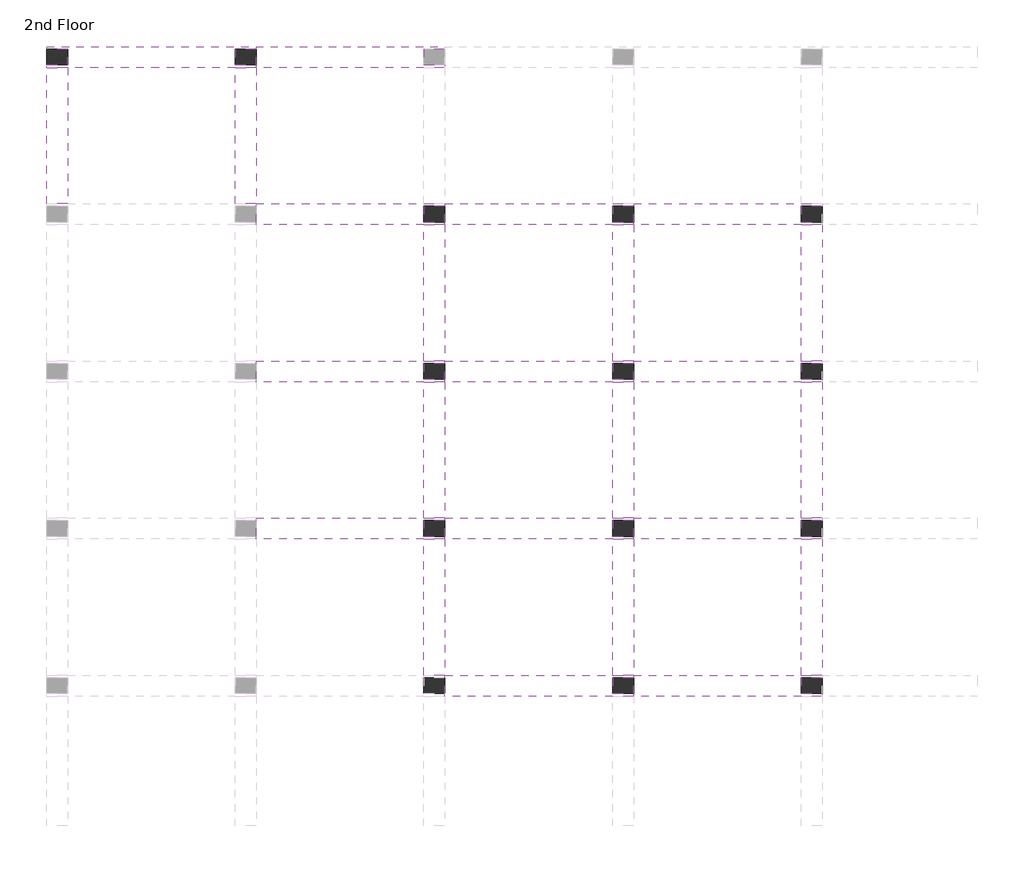
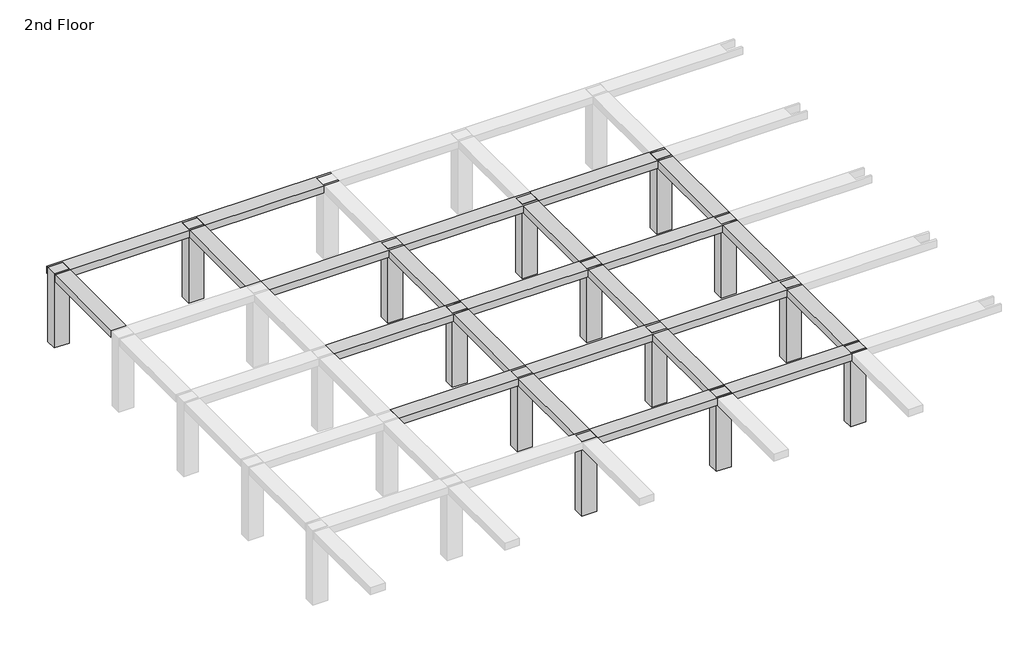
# One storey, part 2 of 3: 24 beams, 14 columns.
"""IFC4 building model written with IfcOpenShell, lengths in millimetres."""

from ifc_helpers import new_model, si_unit, frame, origin, place, context, project, spatial, polyline, outline, extrude, faceted_brep, element, save

model = new_model("IFC4")

# Units and contexts
model_context = context("Model", 3, world=origin())
ifc_project = project(units=[si_unit("LENGTHUNIT", "METRE", prefix="MILLI")], contexts=[model_context])

# Site, building, storey
site = spatial("IfcSite", under=ifc_project)
building = spatial("IfcBuilding", under=site)
storey = spatial("IfcBuildingStorey", under=building, Name="2nd Floor", Elevation=6400.8)

# Beams
placement = place(None, origin())
element("IfcBeam", 1, ObjectType="Concrete-Rectangular Beam : 2' x2'", at=placement, inside=storey, context=model_context, shape_type="Brep", body=[
    faceted_brep([(-5646.474232, 1680.7831222, 9601.2), (-6256.074232, 1680.7831222, 9601.2), (-11132.874232, 1680.7831222, 9601.2), (-11132.874232, 1604.5831222, 9601.2), (-11132.874232, 1147.3831222, 9601.2), (-11132.874232, 1071.1831222, 9601.2), (-6256.074232, 1071.1831222, 9601.2), (-5646.474232, 1071.1831222, 9601.2), (-5646.474232, 1147.3831222, 9601.2), (-6256.074232, 1147.3831222, 9601.2), (-6256.074232, 1604.5831222, 9601.2), (-5646.474232, 1604.5831222, 9601.2), (-5646.474232, 1071.1831222, 9296.4), (-11132.874232, 1071.1831222, 9296.4), (-6256.074232, 1071.1831222, 9296.4), (-11132.874232, 1147.3831222, 9296.4), (-11132.874232, 1604.5831222, 9296.4), (-11132.874232, 1680.7831222, 9296.4), (-6256.074232, 1680.7831222, 9296.4), (-5646.474232, 1680.7831222, 9296.4), (-5646.474232, 1604.5831222, 9296.4), (-6256.074232, 1604.5831222, 9296.4), (-6256.074232, 1147.3831222, 9296.4), (-5646.474232, 1147.3831222, 9296.4)], [[[0, 1, 2, 3, 4, 5, 6, 7, 8, 9, 10, 11]], [[12, 7, 6, 5, 13, 14]], [[12, 14, 13, 15, 16, 17, 18, 19, 20, 21, 22, 23]], [[0, 19, 18, 17, 2, 1]], [[7, 12, 23, 8]], [[5, 4, 3, 2, 17, 16, 15, 13]], [[22, 9, 8, 23]], [[9, 22, 21, 10]], [[10, 21, 20, 11]], [[19, 0, 11, 20]]]),
])
element("IfcBeam", 2, ObjectType="Concrete-Rectangular Beam : 2' x2'", at=placement, inside=storey, context=model_context, shape_type="Brep", body=[
    faceted_brep([(-5646.474232, 1680.7831222, 9601.2), (-5646.474232, 1604.5831222, 9601.2), (-5646.474232, 1147.3831222, 9601.2), (-5646.474232, 1071.1831222, 9601.2), (-769.674232, 1071.1831222, 9601.2), (-160.074232, 1071.1831222, 9601.2), (-160.074232, 1147.3831222, 9601.2), (-769.674232, 1147.3831222, 9601.2), (-769.674232, 1604.5831222, 9601.2), (-160.074232, 1604.5831222, 9601.2), (-160.074232, 1680.7831222, 9601.2), (-769.674232, 1680.7831222, 9601.2), (-5646.474232, 1071.1831222, 9296.4), (-769.674232, 1071.1831222, 9296.4), (-160.074232, 1071.1831222, 9296.4), (-5646.474232, 1147.3831222, 9296.4), (-5646.474232, 1604.5831222, 9296.4), (-5646.474232, 1680.7831222, 9296.4), (-769.674232, 1680.7831222, 9296.4), (-160.074232, 1680.7831222, 9296.4), (-160.074232, 1604.5831222, 9296.4), (-769.674232, 1604.5831222, 9296.4), (-769.674232, 1147.3831222, 9296.4), (-160.074232, 1147.3831222, 9296.4)], [[[0, 1, 2, 3, 4, 5, 6, 7, 8, 9, 10, 11]], [[3, 12, 13, 14, 5, 4]], [[12, 15, 16, 17, 18, 19, 20, 21, 22, 23, 14, 13]], [[10, 19, 18, 17, 0, 11]], [[3, 2, 1, 0, 17, 16, 15, 12]], [[5, 14, 23, 6]], [[22, 7, 6, 23]], [[7, 22, 21, 8]], [[8, 21, 20, 9]], [[19, 10, 9, 20]]]),
])
element("IfcBeam", 3, ObjectType="Concrete-Rectangular Beam : 2' x2'", at=placement, inside=storey, context=model_context, shape_type="Brep", body=[
    faceted_brep([(-16619.274232, 6252.7831222, 9601.2), (-16619.274232, 6176.5831222, 9601.2), (-16619.274232, 5719.3831222, 9601.2), (-16619.274232, 5643.1831222, 9601.2), (-11742.474232, 5643.1831222, 9601.2), (-11132.874232, 5643.1831222, 9601.2), (-11132.874232, 5719.3831222, 9601.2), (-11742.474232, 5719.3831222, 9601.2), (-11742.474232, 6176.5831222, 9601.2), (-11132.874232, 6176.5831222, 9601.2), (-11132.874232, 6252.7831222, 9601.2), (-11742.474232, 6252.7831222, 9601.2), (-16619.274232, 5643.1831222, 9296.4), (-11742.474232, 5643.1831222, 9296.4), (-11132.874232, 5643.1831222, 9296.4), (-16619.274232, 5719.3831222, 9296.4), (-16619.274232, 6176.5831222, 9296.4), (-16619.274232, 6252.7831222, 9296.4), (-11742.474232, 6252.7831222, 9296.4), (-11132.874232, 6252.7831222, 9296.4), (-11132.874232, 6176.5831222, 9296.4), (-11742.474232, 6176.5831222, 9296.4), (-11742.474232, 5719.3831222, 9296.4), (-11132.874232, 5719.3831222, 9296.4)], [[[0, 1, 2, 3, 4, 5, 6, 7, 8, 9, 10, 11]], [[3, 12, 13, 14, 5, 4]], [[12, 15, 16, 17, 18, 19, 20, 21, 22, 23, 14, 13]], [[10, 19, 18, 17, 0, 11]], [[3, 2, 1, 0, 17, 16, 15, 12]], [[5, 14, 23, 6]], [[22, 7, 6, 23]], [[7, 22, 21, 8]], [[8, 21, 20, 9]], [[19, 10, 9, 20]]]),
])
element("IfcBeam", 4, ObjectType="Concrete-Rectangular Beam : 2' x2'", at=placement, inside=storey, context=model_context, shape_type="Brep", body=[
    faceted_brep([(-5646.474232, 6252.7831222, 9601.2), (-6256.074232, 6252.7831222, 9601.2), (-11132.874232, 6252.7831222, 9601.2), (-11132.874232, 6176.5831222, 9601.2), (-11132.874232, 5719.3831222, 9601.2), (-11132.874232, 5643.1831222, 9601.2), (-6256.074232, 5643.1831222, 9601.2), (-5646.474232, 5643.1831222, 9601.2), (-5646.474232, 5719.3831222, 9601.2), (-6256.074232, 5719.3831222, 9601.2), (-6256.074232, 6176.5831222, 9601.2), (-5646.474232, 6176.5831222, 9601.2), (-5646.474232, 5643.1831222, 9296.4), (-11132.874232, 5643.1831222, 9296.4), (-6256.074232, 5643.1831222, 9296.4), (-11132.874232, 5719.3831222, 9296.4), (-11132.874232, 6176.5831222, 9296.4), (-11132.874232, 6252.7831222, 9296.4), (-6256.074232, 6252.7831222, 9296.4), (-5646.474232, 6252.7831222, 9296.4), (-5646.474232, 6176.5831222, 9296.4), (-6256.074232, 6176.5831222, 9296.4), (-6256.074232, 5719.3831222, 9296.4), (-5646.474232, 5719.3831222, 9296.4)], [[[0, 1, 2, 3, 4, 5, 6, 7, 8, 9, 10, 11]], [[12, 7, 6, 5, 13, 14]], [[12, 14, 13, 15, 16, 17, 18, 19, 20, 21, 22, 23]], [[0, 19, 18, 17, 2, 1]], [[7, 12, 23, 8]], [[5, 4, 3, 2, 17, 16, 15, 13]], [[22, 9, 8, 23]], [[9, 22, 21, 10]], [[10, 21, 20, 11]], [[19, 0, 11, 20]]]),
])
element("IfcBeam", 5, ObjectType="Concrete-Rectangular Beam : 2' x2'", at=placement, inside=storey, context=model_context, shape_type="Brep", body=[
    faceted_brep([(-5646.474232, 6252.7831222, 9601.2), (-5646.474232, 6176.5831222, 9601.2), (-5646.474232, 5719.3831222, 9601.2), (-5646.474232, 5643.1831222, 9601.2), (-769.674232, 5643.1831222, 9601.2), (-160.074232, 5643.1831222, 9601.2), (-160.074232, 5719.3831222, 9601.2), (-769.674232, 5719.3831222, 9601.2), (-769.674232, 6176.5831222, 9601.2), (-160.074232, 6176.5831222, 9601.2), (-160.074232, 6252.7831222, 9601.2), (-769.674232, 6252.7831222, 9601.2), (-5646.474232, 5643.1831222, 9296.4), (-769.674232, 5643.1831222, 9296.4), (-160.074232, 5643.1831222, 9296.4), (-5646.474232, 5719.3831222, 9296.4), (-5646.474232, 6176.5831222, 9296.4), (-5646.474232, 6252.7831222, 9296.4), (-769.674232, 6252.7831222, 9296.4), (-160.074232, 6252.7831222, 9296.4), (-160.074232, 6176.5831222, 9296.4), (-769.674232, 6176.5831222, 9296.4), (-769.674232, 5719.3831222, 9296.4), (-160.074232, 5719.3831222, 9296.4)], [[[0, 1, 2, 3, 4, 5, 6, 7, 8, 9, 10, 11]], [[3, 12, 13, 14, 5, 4]], [[12, 15, 16, 17, 18, 19, 20, 21, 22, 23, 14, 13]], [[10, 19, 18, 17, 0, 11]], [[3, 2, 1, 0, 17, 16, 15, 12]], [[5, 14, 23, 6]], [[22, 7, 6, 23]], [[7, 22, 21, 8]], [[8, 21, 20, 9]], [[19, 10, 9, 20]]]),
])
element("IfcBeam", 6, ObjectType="Concrete-Rectangular Beam : 2' x2'", at=placement, inside=storey, context=model_context, shape_type="Brep", body=[
    faceted_brep([(-16619.274232, 10824.7831222, 9601.2), (-16619.274232, 10748.5831222, 9601.2), (-16619.274232, 10291.3831222, 9601.2), (-16619.274232, 10215.1831222, 9601.2), (-11742.474232, 10215.1831222, 9601.2), (-11132.874232, 10215.1831222, 9601.2), (-11132.874232, 10291.3831222, 9601.2), (-11742.474232, 10291.3831222, 9601.2), (-11742.474232, 10748.5831222, 9601.2), (-11132.874232, 10748.5831222, 9601.2), (-11132.874232, 10824.7831222, 9601.2), (-11742.474232, 10824.7831222, 9601.2), (-16619.274232, 10215.1831222, 9296.4), (-11742.474232, 10215.1831222, 9296.4), (-11132.874232, 10215.1831222, 9296.4), (-16619.274232, 10291.3831222, 9296.4), (-16619.274232, 10748.5831222, 9296.4), (-16619.274232, 10824.7831222, 9296.4), (-11742.474232, 10824.7831222, 9296.4), (-11132.874232, 10824.7831222, 9296.4), (-11132.874232, 10748.5831222, 9296.4), (-11742.474232, 10748.5831222, 9296.4), (-11742.474232, 10291.3831222, 9296.4), (-11132.874232, 10291.3831222, 9296.4)], [[[0, 1, 2, 3, 4, 5, 6, 7, 8, 9, 10, 11]], [[3, 12, 13, 14, 5, 4]], [[12, 15, 16, 17, 18, 19, 20, 21, 22, 23, 14, 13]], [[10, 19, 18, 17, 0, 11]], [[3, 2, 1, 0, 17, 16, 15, 12]], [[5, 14, 23, 6]], [[22, 7, 6, 23]], [[7, 22, 21, 8]], [[8, 21, 20, 9]], [[19, 10, 9, 20]]]),
])
element("IfcBeam", 7, ObjectType="Concrete-Rectangular Beam : 2' x2'", at=placement, inside=storey, context=model_context, shape_type="Brep", body=[
    faceted_brep([(-11132.874232, 10824.7831222, 9601.2), (-11132.874232, 10748.5831222, 9601.2), (-11132.874232, 10291.3831222, 9601.2), (-11132.874232, 10215.1831222, 9601.2), (-6256.074232, 10215.1831222, 9601.2), (-5646.474232, 10215.1831222, 9601.2), (-5646.474232, 10291.3831222, 9601.2), (-6256.074232, 10291.3831222, 9601.2), (-6256.074232, 10748.5831222, 9601.2), (-5646.474232, 10748.5831222, 9601.2), (-5646.474232, 10824.7831222, 9601.2), (-6256.074232, 10824.7831222, 9601.2), (-11132.874232, 10215.1831222, 9296.4), (-6256.074232, 10215.1831222, 9296.4), (-5646.474232, 10215.1831222, 9296.4), (-11132.874232, 10291.3831222, 9296.4), (-11132.874232, 10748.5831222, 9296.4), (-11132.874232, 10824.7831222, 9296.4), (-6256.074232, 10824.7831222, 9296.4), (-5646.474232, 10824.7831222, 9296.4), (-5646.474232, 10748.5831222, 9296.4), (-6256.074232, 10748.5831222, 9296.4), (-6256.074232, 10291.3831222, 9296.4), (-5646.474232, 10291.3831222, 9296.4)], [[[0, 1, 2, 3, 4, 5, 6, 7, 8, 9, 10, 11]], [[3, 12, 13, 14, 5, 4]], [[12, 15, 16, 17, 18, 19, 20, 21, 22, 23, 14, 13]], [[10, 19, 18, 17, 0, 11]], [[3, 2, 1, 0, 17, 16, 15, 12]], [[5, 14, 23, 6]], [[22, 7, 6, 23]], [[7, 22, 21, 8]], [[8, 21, 20, 9]], [[19, 10, 9, 20]]]),
])
element("IfcBeam", 8, ObjectType="Concrete-Rectangular Beam : 2' x2'", at=placement, inside=storey, context=model_context, shape_type="Brep", body=[
    faceted_brep([(-5646.474232, 10824.7831222, 9601.2), (-5646.474232, 10748.5831222, 9601.2), (-5646.474232, 10291.3831222, 9601.2), (-5646.474232, 10215.1831222, 9601.2), (-769.674232, 10215.1831222, 9601.2), (-160.074232, 10215.1831222, 9601.2), (-160.074232, 10291.3831222, 9601.2), (-769.674232, 10291.3831222, 9601.2), (-769.674232, 10748.5831222, 9601.2), (-160.074232, 10748.5831222, 9601.2), (-160.074232, 10824.7831222, 9601.2), (-769.674232, 10824.7831222, 9601.2), (-5646.474232, 10215.1831222, 9296.4), (-769.674232, 10215.1831222, 9296.4), (-160.074232, 10215.1831222, 9296.4), (-5646.474232, 10291.3831222, 9296.4), (-5646.474232, 10748.5831222, 9296.4), (-5646.474232, 10824.7831222, 9296.4), (-769.674232, 10824.7831222, 9296.4), (-160.074232, 10824.7831222, 9296.4), (-160.074232, 10748.5831222, 9296.4), (-769.674232, 10748.5831222, 9296.4), (-769.674232, 10291.3831222, 9296.4), (-160.074232, 10291.3831222, 9296.4)], [[[0, 1, 2, 3, 4, 5, 6, 7, 8, 9, 10, 11]], [[3, 12, 13, 14, 5, 4]], [[12, 15, 16, 17, 18, 19, 20, 21, 22, 23, 14, 13]], [[10, 19, 18, 17, 0, 11]], [[3, 2, 1, 0, 17, 16, 15, 12]], [[5, 14, 23, 6]], [[22, 7, 6, 23]], [[7, 22, 21, 8]], [[8, 21, 20, 9]], [[19, 10, 9, 20]]]),
])
element("IfcBeam", 9, ObjectType="Concrete-Rectangular Beam : 2' x2'", at=placement, inside=storey, context=model_context, shape_type="Brep", body=[
    faceted_brep([(-16619.274232, 15396.7831222, 9601.2), (-16619.274232, 15320.5831222, 9601.2), (-16619.274232, 14863.3831222, 9601.2), (-16619.274232, 14787.1831222, 9601.2), (-11742.474232, 14787.1831222, 9601.2), (-11132.874232, 14787.1831222, 9601.2), (-11132.874232, 14863.3831222, 9601.2), (-11742.474232, 14863.3831222, 9601.2), (-11742.474232, 15320.5831222, 9601.2), (-11132.874232, 15320.5831222, 9601.2), (-11132.874232, 15396.7831222, 9601.2), (-11742.474232, 15396.7831222, 9601.2), (-16619.274232, 14787.1831222, 9296.4), (-11742.474232, 14787.1831222, 9296.4), (-11132.874232, 14787.1831222, 9296.4), (-16619.274232, 14863.3831222, 9296.4), (-16619.274232, 15320.5831222, 9296.4), (-16619.274232, 15396.7831222, 9296.4), (-11742.474232, 15396.7831222, 9296.4), (-11132.874232, 15396.7831222, 9296.4), (-11132.874232, 15320.5831222, 9296.4), (-11742.474232, 15320.5831222, 9296.4), (-11742.474232, 14863.3831222, 9296.4), (-11132.874232, 14863.3831222, 9296.4)], [[[0, 1, 2, 3, 4, 5, 6, 7, 8, 9, 10, 11]], [[3, 12, 13, 14, 5, 4]], [[12, 15, 16, 17, 18, 19, 20, 21, 22, 23, 14, 13]], [[10, 19, 18, 17, 0, 11]], [[3, 2, 1, 0, 17, 16, 15, 12]], [[5, 14, 23, 6]], [[22, 7, 6, 23]], [[7, 22, 21, 8]], [[8, 21, 20, 9]], [[19, 10, 9, 20]]]),
])
element("IfcBeam", 10, ObjectType="Concrete-Rectangular Beam : 2' x2'", at=placement, inside=storey, context=model_context, shape_type="Brep", body=[
    faceted_brep([(-11132.874232, 15396.7831222, 9601.2), (-11132.874232, 15320.5831222, 9601.2), (-11132.874232, 14863.3831222, 9601.2), (-11132.874232, 14787.1831222, 9601.2), (-6256.074232, 14787.1831222, 9601.2), (-5646.474232, 14787.1831222, 9601.2), (-5646.474232, 14863.3831222, 9601.2), (-6256.074232, 14863.3831222, 9601.2), (-6256.074232, 15320.5831222, 9601.2), (-5646.474232, 15320.5831222, 9601.2), (-5646.474232, 15396.7831222, 9601.2), (-6256.074232, 15396.7831222, 9601.2), (-11132.874232, 14787.1831222, 9296.4), (-6256.074232, 14787.1831222, 9296.4), (-5646.474232, 14787.1831222, 9296.4), (-11132.874232, 14863.3831222, 9296.4), (-11132.874232, 15320.5831222, 9296.4), (-11132.874232, 15396.7831222, 9296.4), (-6256.074232, 15396.7831222, 9296.4), (-5646.474232, 15396.7831222, 9296.4), (-5646.474232, 15320.5831222, 9296.4), (-6256.074232, 15320.5831222, 9296.4), (-6256.074232, 14863.3831222, 9296.4), (-5646.474232, 14863.3831222, 9296.4)], [[[0, 1, 2, 3, 4, 5, 6, 7, 8, 9, 10, 11]], [[3, 12, 13, 14, 5, 4]], [[12, 15, 16, 17, 18, 19, 20, 21, 22, 23, 14, 13]], [[10, 19, 18, 17, 0, 11]], [[3, 2, 1, 0, 17, 16, 15, 12]], [[5, 14, 23, 6]], [[22, 7, 6, 23]], [[7, 22, 21, 8]], [[8, 21, 20, 9]], [[19, 10, 9, 20]]]),
])
element("IfcBeam", 11, ObjectType="Concrete-Rectangular Beam : 2' x2'", at=placement, inside=storey, context=model_context, shape_type="Brep", body=[
    faceted_brep([(-5646.474232, 15396.7831222, 9601.2), (-5646.474232, 15320.5831222, 9601.2), (-5646.474232, 14863.3831222, 9601.2), (-5646.474232, 14787.1831222, 9601.2), (-769.674232, 14787.1831222, 9601.2), (-160.074232, 14787.1831222, 9601.2), (-160.074232, 14863.3831222, 9601.2), (-769.674232, 14863.3831222, 9601.2), (-769.674232, 15320.5831222, 9601.2), (-160.074232, 15320.5831222, 9601.2), (-160.074232, 15396.7831222, 9601.2), (-769.674232, 15396.7831222, 9601.2), (-5646.474232, 14787.1831222, 9296.4), (-769.674232, 14787.1831222, 9296.4), (-160.074232, 14787.1831222, 9296.4), (-5646.474232, 14863.3831222, 9296.4), (-5646.474232, 15320.5831222, 9296.4), (-5646.474232, 15396.7831222, 9296.4), (-769.674232, 15396.7831222, 9296.4), (-160.074232, 15396.7831222, 9296.4), (-160.074232, 15320.5831222, 9296.4), (-769.674232, 15320.5831222, 9296.4), (-769.674232, 14863.3831222, 9296.4), (-160.074232, 14863.3831222, 9296.4)], [[[0, 1, 2, 3, 4, 5, 6, 7, 8, 9, 10, 11]], [[3, 12, 13, 14, 5, 4]], [[12, 15, 16, 17, 18, 19, 20, 21, 22, 23, 14, 13]], [[10, 19, 18, 17, 0, 11]], [[3, 2, 1, 0, 17, 16, 15, 12]], [[5, 14, 23, 6]], [[22, 7, 6, 23]], [[7, 22, 21, 8]], [[8, 21, 20, 9]], [[19, 10, 9, 20]]]),
])
element("IfcBeam", 12, ObjectType="Concrete-Rectangular Beam : 2' x2'", at=placement, inside=storey, context=model_context, shape_type="Brep", body=[
    faceted_brep([(-16619.274232, 19968.7831222, 9601.2), (-22715.274232, 19968.7831222, 9601.2), (-22715.274232, 19892.5831222, 9601.2), (-22105.674232, 19892.5831222, 9601.2), (-22105.674232, 19435.3831222, 9601.2), (-22715.274232, 19435.3831222, 9601.2), (-22715.274232, 19359.1831222, 9601.2), (-22105.674232, 19359.1831222, 9601.2), (-17228.874232, 19359.1831222, 9601.2), (-16619.274232, 19359.1831222, 9601.2), (-16619.274232, 19435.3831222, 9601.2), (-17228.874232, 19435.3831222, 9601.2), (-17228.874232, 19892.5831222, 9601.2), (-16619.274232, 19892.5831222, 9601.2), (-22715.274232, 19359.1831222, 9296.4), (-22105.674232, 19359.1831222, 9296.4), (-17228.874232, 19359.1831222, 9296.4), (-16619.274232, 19359.1831222, 9296.4), (-22715.274232, 19435.3831222, 9296.4), (-22105.674232, 19435.3831222, 9296.4), (-22105.674232, 19892.5831222, 9296.4), (-22715.274232, 19892.5831222, 9296.4), (-22715.274232, 19968.7831222, 9296.4), (-16619.274232, 19968.7831222, 9296.4), (-16619.274232, 19892.5831222, 9296.4), (-17228.874232, 19892.5831222, 9296.4), (-17228.874232, 19435.3831222, 9296.4), (-16619.274232, 19435.3831222, 9296.4)], [[[0, 1, 2, 3, 4, 5, 6, 7, 8, 9, 10, 11, 12, 13]], [[6, 14, 15, 16, 17, 9, 8, 7]], [[17, 16, 15, 14, 18, 19, 20, 21, 22, 23, 24, 25, 26, 27]], [[22, 1, 0, 23]], [[14, 6, 5, 18]], [[9, 17, 27, 10]], [[19, 4, 3, 20]], [[4, 19, 18, 5]], [[20, 3, 2, 21]], [[1, 22, 21, 2]], [[26, 11, 10, 27]], [[11, 26, 25, 12]], [[12, 25, 24, 13]], [[23, 0, 13, 24]]]),
])
element("IfcBeam", 13, ObjectType="Concrete-Rectangular Beam : 2' x2'", at=placement, inside=storey, context=model_context, shape_type="Brep", body=[
    faceted_brep([(-11132.874232, 19968.7831222, 9601.2), (-16619.274232, 19968.7831222, 9601.2), (-16619.274232, 19892.5831222, 9601.2), (-16619.274232, 19435.3831222, 9601.2), (-16619.274232, 19359.1831222, 9601.2), (-11742.474232, 19359.1831222, 9601.2), (-11132.874232, 19359.1831222, 9601.2), (-11132.874232, 19435.3831222, 9601.2), (-11742.474232, 19435.3831222, 9601.2), (-11742.474232, 19892.5831222, 9601.2), (-11132.874232, 19892.5831222, 9601.2), (-11132.874232, 19359.1831222, 9296.4), (-16619.274232, 19359.1831222, 9296.4), (-11742.474232, 19359.1831222, 9296.4), (-16619.274232, 19435.3831222, 9296.4), (-16619.274232, 19892.5831222, 9296.4), (-16619.274232, 19968.7831222, 9296.4), (-11132.874232, 19968.7831222, 9296.4), (-11132.874232, 19892.5831222, 9296.4), (-11742.474232, 19892.5831222, 9296.4), (-11742.474232, 19435.3831222, 9296.4), (-11132.874232, 19435.3831222, 9296.4)], [[[0, 1, 2, 3, 4, 5, 6, 7, 8, 9, 10]], [[11, 6, 5, 4, 12, 13]], [[11, 13, 12, 14, 15, 16, 17, 18, 19, 20, 21]], [[0, 17, 16, 1]], [[6, 11, 21, 7]], [[4, 3, 2, 1, 16, 15, 14, 12]], [[20, 8, 7, 21]], [[8, 20, 19, 9]], [[9, 19, 18, 10]], [[17, 0, 10, 18]]]),
])
element("IfcBeam", 14, ObjectType="Concrete-Rectangular Beam : 2' x2'", at=placement, inside=storey, context=model_context, shape_type="SweptSolid", body=[
    extrude(outline(polyline([(-22105.674232, 15396.7831222), (-22715.274232, 15396.7831222), (-22715.274232, 19359.1831222), (-22105.674232, 19359.1831222), (-22105.674232, 15396.7831222)])), frame((0.0, 0.0, 9296.4), z_axis=(0.0, 0.0, 1.0), x_axis=(1.0, 0.0, 0.0)), (0.0, 0.0, 1.0), 304.8),
])
element("IfcBeam", 15, ObjectType="Concrete-Rectangular Beam : 2' x2'", at=placement, inside=storey, context=model_context, shape_type="SweptSolid", body=[
    extrude(outline(polyline([(-16619.274232, 15396.7831222), (-17228.874232, 15396.7831222), (-17228.874232, 19359.1831222), (-16619.274232, 19359.1831222), (-16619.274232, 15396.7831222)])), frame((0.0, 0.0, 9296.4), z_axis=(0.0, 0.0, 1.0), x_axis=(1.0, 0.0, 0.0)), (0.0, 0.0, 1.0), 304.8),
])
element("IfcBeam", 16, ObjectType="Concrete-Rectangular Beam : 2' x2'", at=placement, inside=storey, context=model_context, shape_type="SweptSolid", body=[
    extrude(outline(polyline([(-11132.874232, 1680.7831222), (-11742.474232, 1680.7831222), (-11742.474232, 5643.1831222), (-11132.874232, 5643.1831222), (-11132.874232, 1680.7831222)])), frame((0.0, 0.0, 9296.4), z_axis=(0.0, 0.0, 1.0), x_axis=(1.0, 0.0, 0.0)), (0.0, 0.0, 1.0), 304.8),
])
element("IfcBeam", 17, ObjectType="Concrete-Rectangular Beam : 2' x2'", at=placement, inside=storey, context=model_context, shape_type="SweptSolid", body=[
    extrude(outline(polyline([(-11132.874232, 6252.7831222), (-11742.474232, 6252.7831222), (-11742.474232, 10215.1831222), (-11132.874232, 10215.1831222), (-11132.874232, 6252.7831222)])), frame((0.0, 0.0, 9296.4), z_axis=(0.0, 0.0, 1.0), x_axis=(1.0, 0.0, 0.0)), (0.0, 0.0, 1.0), 304.8),
])
element("IfcBeam", 18, ObjectType="Concrete-Rectangular Beam : 2' x2'", at=placement, inside=storey, context=model_context, shape_type="SweptSolid", body=[
    extrude(outline(polyline([(-11132.874232, 10824.7831222), (-11742.474232, 10824.7831222), (-11742.474232, 14787.1831222), (-11132.874232, 14787.1831222), (-11132.874232, 10824.7831222)])), frame((0.0, 0.0, 9296.4), z_axis=(0.0, 0.0, 1.0), x_axis=(1.0, 0.0, 0.0)), (0.0, 0.0, 1.0), 304.8),
])
element("IfcBeam", 19, ObjectType="Concrete-Rectangular Beam : 2' x2'", at=placement, inside=storey, context=model_context, shape_type="SweptSolid", body=[
    extrude(outline(polyline([(-5646.474232, 1680.7831222), (-6256.074232, 1680.7831222), (-6256.074232, 5643.1831222), (-5646.474232, 5643.1831222), (-5646.474232, 1680.7831222)])), frame((0.0, 0.0, 9296.4), z_axis=(0.0, 0.0, 1.0), x_axis=(1.0, 0.0, 0.0)), (0.0, 0.0, 1.0), 304.8),
])
element("IfcBeam", 20, ObjectType="Concrete-Rectangular Beam : 2' x2'", at=placement, inside=storey, context=model_context, shape_type="SweptSolid", body=[
    extrude(outline(polyline([(-5646.474232, 6252.7831222), (-6256.074232, 6252.7831222), (-6256.074232, 10215.1831222), (-5646.474232, 10215.1831222), (-5646.474232, 6252.7831222)])), frame((0.0, 0.0, 9296.4), z_axis=(0.0, 0.0, 1.0), x_axis=(1.0, 0.0, 0.0)), (0.0, 0.0, 1.0), 304.8),
])
element("IfcBeam", 21, ObjectType="Concrete-Rectangular Beam : 2' x2'", at=placement, inside=storey, context=model_context, shape_type="SweptSolid", body=[
    extrude(outline(polyline([(-5646.474232, 10824.7831222), (-6256.074232, 10824.7831222), (-6256.074232, 14787.1831222), (-5646.474232, 14787.1831222), (-5646.474232, 10824.7831222)])), frame((0.0, 0.0, 9296.4), z_axis=(0.0, 0.0, 1.0), x_axis=(1.0, 0.0, 0.0)), (0.0, 0.0, 1.0), 304.8),
])
element("IfcBeam", 22, ObjectType="Concrete-Rectangular Beam : 2' x2'", at=placement, inside=storey, context=model_context, shape_type="SweptSolid", body=[
    extrude(outline(polyline([(-769.674232, 5643.1831222), (-160.074232, 5643.1831222), (-160.074232, 1680.7831222), (-769.674232, 1680.7831222), (-769.674232, 5643.1831222)])), frame((0.0, 0.0, 9296.4), z_axis=(0.0, 0.0, 1.0), x_axis=(1.0, 0.0, 0.0)), (0.0, 0.0, 1.0), 304.8),
])
element("IfcBeam", 23, ObjectType="Concrete-Rectangular Beam : 2' x2'", at=placement, inside=storey, context=model_context, shape_type="SweptSolid", body=[
    extrude(outline(polyline([(-160.074232, 6252.7831222), (-769.674232, 6252.7831222), (-769.674232, 10215.1831222), (-160.074232, 10215.1831222), (-160.074232, 6252.7831222)])), frame((0.0, 0.0, 9296.4), z_axis=(0.0, 0.0, 1.0), x_axis=(1.0, 0.0, 0.0)), (0.0, 0.0, 1.0), 304.8),
])
element("IfcBeam", 24, ObjectType="Concrete-Rectangular Beam : 2' x2'", at=placement, inside=storey, context=model_context, shape_type="SweptSolid", body=[
    extrude(outline(polyline([(-769.674232, 14787.1831222), (-160.074232, 14787.1831222), (-160.074232, 10824.7831222), (-769.674232, 10824.7831222), (-769.674232, 14787.1831222)])), frame((0.0, 0.0, 9296.4), z_axis=(0.0, 0.0, 1.0), x_axis=(1.0, 0.0, 0.0)), (0.0, 0.0, 1.0), 304.8),
])

# Columns
element("IfcColumn", 25, ObjectType="Concrete-Rectangular-Column : 12 x 18", at=placement, inside=storey, context=model_context, shape_type="SweptSolid", body=[
    extrude(outline(polyline([(-11132.874232, 1604.5831222), (-11132.874232, 1147.3831222), (-11742.474232, 1147.3831222), (-11742.474232, 1604.5831222), (-11132.874232, 1604.5831222)])), frame((0.0, 0.0, 6400.8), z_axis=(0.0, 0.0, 1.0), x_axis=(1.0, 0.0, 0.0)), (0.0, 0.0, 1.0), 3200.4),
])
element("IfcColumn", 26, ObjectType="Concrete-Rectangular-Column : 12 x 18", at=placement, inside=storey, context=model_context, shape_type="SweptSolid", body=[
    extrude(outline(polyline([(-5646.474232, 1604.5831222), (-5646.474232, 1147.3831222), (-6256.074232, 1147.3831222), (-6256.074232, 1604.5831222), (-5646.474232, 1604.5831222)])), frame((0.0, 0.0, 6400.8), z_axis=(0.0, 0.0, 1.0), x_axis=(1.0, 0.0, 0.0)), (0.0, 0.0, 1.0), 3200.4),
])
element("IfcColumn", 27, ObjectType="Concrete-Rectangular-Column : 12 x 18", at=placement, inside=storey, context=model_context, shape_type="SweptSolid", body=[
    extrude(outline(polyline([(-160.074232, 1604.5831222), (-160.074232, 1147.3831222), (-769.674232, 1147.3831222), (-769.674232, 1604.5831222), (-160.074232, 1604.5831222)])), frame((0.0, 0.0, 6400.8), z_axis=(0.0, 0.0, 1.0), x_axis=(1.0, 0.0, 0.0)), (0.0, 0.0, 1.0), 3200.4),
])
element("IfcColumn", 28, ObjectType="Concrete-Rectangular-Column : 12 x 18", at=placement, inside=storey, context=model_context, shape_type="SweptSolid", body=[
    extrude(outline(polyline([(-11132.874232, 6176.5831222), (-11132.874232, 5719.3831222), (-11742.474232, 5719.3831222), (-11742.474232, 6176.5831222), (-11132.874232, 6176.5831222)])), frame((0.0, 0.0, 6400.8), z_axis=(0.0, 0.0, 1.0), x_axis=(1.0, 0.0, 0.0)), (0.0, 0.0, 1.0), 3200.4),
])
element("IfcColumn", 29, ObjectType="Concrete-Rectangular-Column : 12 x 18", at=placement, inside=storey, context=model_context, shape_type="SweptSolid", body=[
    extrude(outline(polyline([(-5646.474232, 6176.5831222), (-5646.474232, 5719.3831222), (-6256.074232, 5719.3831222), (-6256.074232, 6176.5831222), (-5646.474232, 6176.5831222)])), frame((0.0, 0.0, 6400.8), z_axis=(0.0, 0.0, 1.0), x_axis=(1.0, 0.0, 0.0)), (0.0, 0.0, 1.0), 3200.4),
])
element("IfcColumn", 30, ObjectType="Concrete-Rectangular-Column : 12 x 18", at=placement, inside=storey, context=model_context, shape_type="SweptSolid", body=[
    extrude(outline(polyline([(-160.074232, 6176.5831222), (-160.074232, 5719.3831222), (-769.674232, 5719.3831222), (-769.674232, 6176.5831222), (-160.074232, 6176.5831222)])), frame((0.0, 0.0, 6400.8), z_axis=(0.0, 0.0, 1.0), x_axis=(1.0, 0.0, 0.0)), (0.0, 0.0, 1.0), 3200.4),
])
element("IfcColumn", 31, ObjectType="Concrete-Rectangular-Column : 12 x 18", at=placement, inside=storey, context=model_context, shape_type="SweptSolid", body=[
    extrude(outline(polyline([(-11132.874232, 10748.5831222), (-11132.874232, 10291.3831222), (-11742.474232, 10291.3831222), (-11742.474232, 10748.5831222), (-11132.874232, 10748.5831222)])), frame((0.0, 0.0, 6400.8), z_axis=(0.0, 0.0, 1.0), x_axis=(1.0, 0.0, 0.0)), (0.0, 0.0, 1.0), 3200.4),
])
element("IfcColumn", 32, ObjectType="Concrete-Rectangular-Column : 12 x 18", at=placement, inside=storey, context=model_context, shape_type="SweptSolid", body=[
    extrude(outline(polyline([(-5646.474232, 10748.5831222), (-5646.474232, 10291.3831222), (-6256.074232, 10291.3831222), (-6256.074232, 10748.5831222), (-5646.474232, 10748.5831222)])), frame((0.0, 0.0, 6400.8), z_axis=(0.0, 0.0, 1.0), x_axis=(1.0, 0.0, 0.0)), (0.0, 0.0, 1.0), 3200.4),
])
element("IfcColumn", 33, ObjectType="Concrete-Rectangular-Column : 12 x 18", at=placement, inside=storey, context=model_context, shape_type="SweptSolid", body=[
    extrude(outline(polyline([(-160.074232, 10748.5831222), (-160.074232, 10291.3831222), (-769.674232, 10291.3831222), (-769.674232, 10748.5831222), (-160.074232, 10748.5831222)])), frame((0.0, 0.0, 6400.8), z_axis=(0.0, 0.0, 1.0), x_axis=(1.0, 0.0, 0.0)), (0.0, 0.0, 1.0), 3200.4),
])
element("IfcColumn", 34, ObjectType="Concrete-Rectangular-Column : 12 x 18", at=placement, inside=storey, context=model_context, shape_type="SweptSolid", body=[
    extrude(outline(polyline([(-11132.874232, 15320.5831222), (-11132.874232, 14863.3831222), (-11742.474232, 14863.3831222), (-11742.474232, 15320.5831222), (-11132.874232, 15320.5831222)])), frame((0.0, 0.0, 6400.8), z_axis=(0.0, 0.0, 1.0), x_axis=(1.0, 0.0, 0.0)), (0.0, 0.0, 1.0), 3200.4),
])
element("IfcColumn", 35, ObjectType="Concrete-Rectangular-Column : 12 x 18", at=placement, inside=storey, context=model_context, shape_type="SweptSolid", body=[
    extrude(outline(polyline([(-5646.474232, 15320.5831222), (-5646.474232, 14863.3831222), (-6256.074232, 14863.3831222), (-6256.074232, 15320.5831222), (-5646.474232, 15320.5831222)])), frame((0.0, 0.0, 6400.8), z_axis=(0.0, 0.0, 1.0), x_axis=(1.0, 0.0, 0.0)), (0.0, 0.0, 1.0), 3200.4),
])
element("IfcColumn", 36, ObjectType="Concrete-Rectangular-Column : 12 x 18", at=placement, inside=storey, context=model_context, shape_type="SweptSolid", body=[
    extrude(outline(polyline([(-160.074232, 15320.5831222), (-160.074232, 14863.3831222), (-769.674232, 14863.3831222), (-769.674232, 15320.5831222), (-160.074232, 15320.5831222)])), frame((0.0, 0.0, 6400.8), z_axis=(0.0, 0.0, 1.0), x_axis=(1.0, 0.0, 0.0)), (0.0, 0.0, 1.0), 3200.4),
])
element("IfcColumn", 37, ObjectType="Concrete-Rectangular-Column : 12 x 18", at=placement, inside=storey, context=model_context, shape_type="SweptSolid", body=[
    extrude(outline(polyline([(-22105.674232, 19892.5831222), (-22105.674232, 19435.3831222), (-22715.274232, 19435.3831222), (-22715.274232, 19892.5831222), (-22105.674232, 19892.5831222)])), frame((0.0, 0.0, 6400.8), z_axis=(0.0, 0.0, 1.0), x_axis=(1.0, 0.0, 0.0)), (0.0, 0.0, 1.0), 3200.4),
])
element("IfcColumn", 38, ObjectType="Concrete-Rectangular-Column : 12 x 18", at=placement, inside=storey, context=model_context, shape_type="SweptSolid", body=[
    extrude(outline(polyline([(-16619.274232, 19892.5831222), (-16619.274232, 19435.3831222), (-17228.874232, 19435.3831222), (-17228.874232, 19892.5831222), (-16619.274232, 19892.5831222)])), frame((0.0, 0.0, 6400.8), z_axis=(0.0, 0.0, 1.0), x_axis=(1.0, 0.0, 0.0)), (0.0, 0.0, 1.0), 3200.4),
])

save(model, "model.ifc")

# Revit data of these elements
# Type "Concrete-Rectangular Beam : 2' x2'"
#   Assembly Code = "B10"
#   Length [instance default] = 5' - 0"
#   b = 2' - 0"
#   h = 1' - 0"
#   Structural Material [instance default] = Concrete, Cast-in-Place gray
# Type "Concrete-Rectangular-Column : 12 x 18"
#   Assembly Code = "B10"
#   b = 2' - 0"
#   h = 1' - 6"
#   Structural Material [instance default] = Concrete, Cast-in-Place gray
# Elements 1, 2, 3, 4, 5, 6, 7, 8, 9, 10, 11, 12, 13, 14, 15, 16, 17, 18, 19, 20, 21, 22, 23, 24 (IfcBeam, "Concrete-Rectangular Beam : 2' x2'")
#   Structural Material = Concrete, Precast (2)
#   Phase Created = New Construction
#   Materials on its faces: "Concrete, Precast (2)"
# Elements 25, 26, 27, 28, 29, 30, 31, 32, 33, 34, 35, 36, 37, 38 (IfcColumn, "Concrete-Rectangular-Column : 12 x 18")
#   Phase Created = New Construction
#   Materials on its faces: "Concrete, Cast-in-Place gray"
# Materials
#   "Concrete, Cast-in-Place gray": class "Concrete", colour RGB 192 192 192, transparency 0, Description = "Cast-in-place concrete", Cost = 0
#   "Concrete, Precast (2)": class "Concrete", colour RGB 198 187 187, transparency 0, Description = "Precast concrete", Cost = 0
